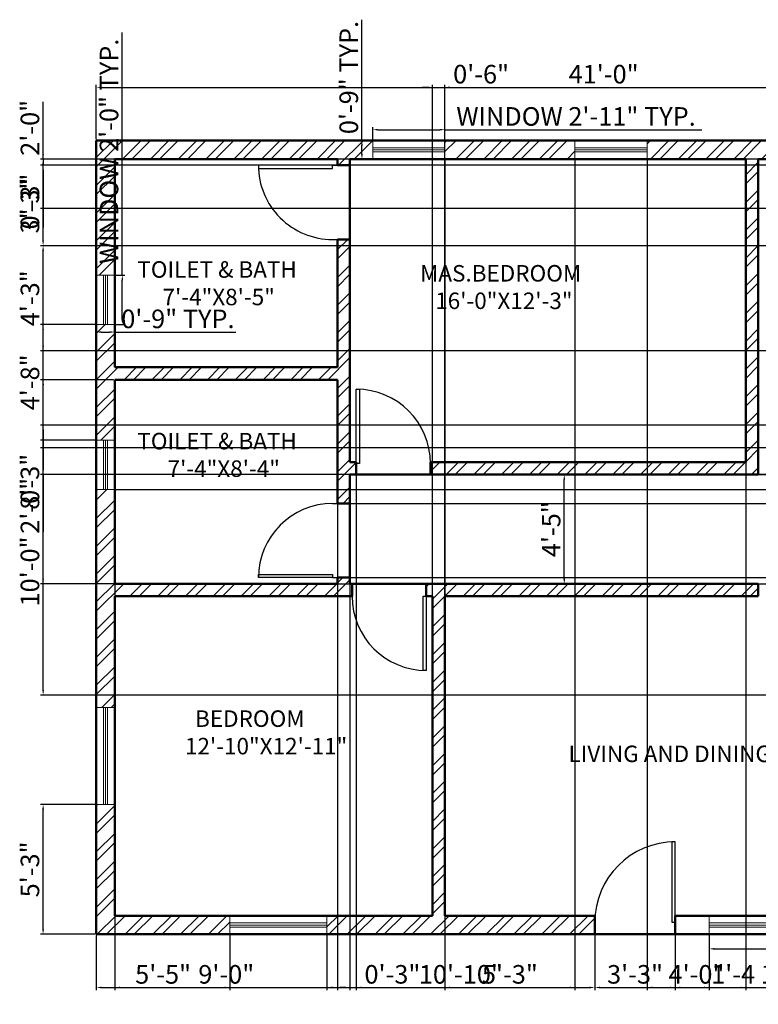
# Model space of a CAD drawing. Units: inches. Extents: x 935 to 4718, y 294 to 2318.
# Tile 1 of 2: x 935 to 1293, y 1841 to 2318. Entities that reach past the tile are written whole.
import ezdxf

# ---------------------------------------------------------------- set-up
doc = ezdxf.new("R2010")
doc.units = ezdxf.units.IN
for name, color, linetype, lineweight in [('A-ANNO-DIMS', 2, 'Continuous', 18), ('A-AREA-IDEN', 7, 'Continuous', 25), ('A-DOOR', 4, 'Continuous', 25), ('A-FLOR-CASE', 8, 'Continuous', 25), ('A-GLAZ', 244, 'Continuous', 18), ('A-WALL', 7, 'Continuous', 50), ('A-WALL-PATT', 8, 'Continuous', 13)]:
    doc.layers.add(name, color=color, linetype=linetype, lineweight=lineweight)
doc.styles.get("Standard").update_dxf_attribs({"font": 'arial.ttf'})
doc.dimstyles.new('ISO-25', dxfattribs={"dimtxt": 9, "dimasz": 2.5, "dimexe": 1.25, "dimexo": 0.625, "dimtad": 1, "dimlunit": 3, "dimtxsty": 'Standard', "dimcen": 2.5, "dimadec": 0, "dimazin": 0, "dimtfac": 1, "dimtmove": 0, "dimatfit": 3, "dimfxl": 1, "dimarcsym": 0})

# ---------------------------------------------------------------- blocks, each defined once
blk = doc.blocks.new('*U2')
for p, q in [((0, 0), (0, -6)), ((40, 0), (40, -6))]:
    blk.add_line(p, q)
blk.add_lwpolyline([(0, 0), (0, 40), (1.75, 40), (1.75, 0)], close=True)
blk.add_arc((0, 0), 40, 0, 90)
blk = doc.blocks.new('*U3')
for p, q in [((0, 0), (0, -6)), ((-40, 0), (-40, -6))]:
    blk.add_line(p, q)
blk.add_lwpolyline([(0, 0), (0, 40), (-1.75, 40), (-1.75, 0)], close=True)
blk.add_arc((0, 0), 40, 90, 180)
blk = doc.blocks.new('*U4')
for p, q in [((-40, 0), (-40, 6)), ((0, 0), (0, 6))]:
    blk.add_line(p, q)
blk.add_lwpolyline([(0, 0), (0, -40), (-1.75, -40), (-1.75, 0)], close=True)
blk.add_arc((0, 0), 40, 180, 270)
blk = doc.blocks.new('*U5')
for p, q in [((0, 0), (0, 6)), ((40, 0), (40, 6))]:
    blk.add_line(p, q)
blk.add_lwpolyline([(0, 0), (0, -40), (1.75, -40), (1.75, 0)], close=True)
blk.add_arc((0, 0), 40, 270, 0)
blk = doc.blocks.new('*D6')
at = {"layer": 'A-ANNO-DIMS', "color": 0, "lineweight": -2, "transparency": 16777216}
for p, q in [((1201.5, 2097.69), (1197.39, 2097.69)), ((1198.64, 2047.19), (1198.64, 2095.19)), ((1201.5, 2044.69), (1197.39, 2044.69))]:
    blk.add_line(p, q, dxfattribs=at)
at = {"layer": 'A-ANNO-DIMS', "color": 0, "transparency": 16777216}
for points in [[(1198.22, 2095.19), (1199.06, 2095.19), (1198.64, 2097.69)], [(1198.22, 2047.19), (1199.06, 2047.19), (1198.64, 2044.69)]]:
    blk.add_solid(points, dxfattribs=at)
at = {"layer": 'Defpoints', "color": 0, "transparency": 16777216}
for p in [(1198.64, 2097.69), (1202.12, 2097.69), (1202.12, 2044.69)]:
    blk.add_point(p, dxfattribs=at)
at = {"layer": 'A-ANNO-DIMS', "color": 0, "transparency": 16777216, "insert": (1193.44, 2071.19), "char_height": 9, "attachment_point": 5, "rotation": 90}
blk.add_mtext('4\'-5"', dxfattribs=at)
blk = doc.blocks.new('WIN-47IN')
for p, q in [((0, 5.5), (47, 5.5)), ((0, 4.5), (47, 4.5)), ((0, 3.5), (47, 3.5))]:
    blk.add_line(p, q)
blk.add_lwpolyline([(0, 9), (47, 9), (47, 0), (0, 0)], close=True)
blk = doc.blocks.new('WIN-35IN')
for p, q in [((0, 5.5), (35, 5.5)), ((0, 4.5), (35, 4.5)), ((0, 3.5), (35, 3.5))]:
    blk.add_line(p, q)
blk.add_lwpolyline([(0, 9), (35, 9), (35, 0), (0, 0)], close=True)
blk = doc.blocks.new('WIN-24IN')
for p, q in [((3.5, 24), (3.5, 0)), ((4.5, 24), (4.5, 0)), ((5.5, 24), (5.5, 0))]:
    blk.add_line(p, q)
blk.add_lwpolyline([(0, 24), (9, 24), (9, 0), (0, 0)], close=True)
blk = doc.blocks.new('*D10')
at = {"layer": 'A-ANNO-DIMS', "color": 0, "lineweight": -2, "transparency": 16777216}
for p, q in [((1268.86, 1874.07), (1268.86, 1866.39)), ((1315.86, 1874.07), (1315.86, 1866.39)), ((1271.36, 1867.64), (1313.36, 1867.64)), ((1315.86, 1867.64), (1440.49, 1867.64))]:
    blk.add_line(p, q, dxfattribs=at)
at = {"layer": 'A-ANNO-DIMS', "color": 0, "transparency": 16777216}
for points in [[(1271.36, 1868.06), (1271.36, 1867.23), (1268.86, 1867.64)], [(1313.36, 1868.06), (1313.36, 1867.23), (1315.86, 1867.64)]]:
    blk.add_solid(points, dxfattribs=at)
at = {"layer": 'Defpoints', "color": 0, "transparency": 16777216}
for p in [(1268.86, 1874.69), (1315.86, 1874.69), (1315.86, 1867.64)]:
    blk.add_point(p, dxfattribs=at)
at = {"layer": 'A-ANNO-DIMS', "color": 0, "transparency": 16777216, "insert": (1379.42, 1872.93), "char_height": 9, "attachment_point": 5}
blk.add_mtext('WINDOW 3\'-11" TYP.', dxfattribs=at)
blk = doc.blocks.new('*D12')
at = {"layer": 'A-ANNO-DIMS', "color": 0, "lineweight": -2, "transparency": 16777216}
for p, q in [((1105.77, 2260.32), (1105.77, 2266.19)), ((1108.27, 2264.94), (1138.27, 2264.94)), ((1140.77, 2260.32), (1140.77, 2266.19)), ((1140.77, 2264.94), (1265.4, 2264.94))]:
    blk.add_line(p, q, dxfattribs=at)
at = {"layer": 'A-ANNO-DIMS', "color": 0, "transparency": 16777216}
for points in [[(1108.27, 2265.36), (1108.27, 2264.53), (1105.77, 2264.94)], [(1138.27, 2265.36), (1138.27, 2264.53), (1140.77, 2264.94)]]:
    blk.add_solid(points, dxfattribs=at)
at = {"layer": 'Defpoints', "color": 0, "transparency": 16777216}
for p in [(1140.77, 2264.94), (1105.77, 2259.69), (1140.77, 2259.69)]:
    blk.add_point(p, dxfattribs=at)
at = {"layer": 'A-ANNO-DIMS', "color": 0, "transparency": 16777216, "insert": (1204.34, 2270.22), "char_height": 9, "attachment_point": 5}
blk.add_mtext('WINDOW 2\'-11" TYP.', dxfattribs=at)
blk = doc.blocks.new('*D13')
at = {"layer": 'A-ANNO-DIMS', "color": 0, "lineweight": -2, "transparency": 16777216}
for p, q in [((1100.52, 2259.69), (1100.52, 2318.3)), ((1105.15, 2259.69), (1099.27, 2259.69)), ((1100.52, 2253.19), (1100.52, 2257.19)), ((1105.15, 2250.69), (1099.27, 2250.69))]:
    blk.add_line(p, q, dxfattribs=at)
at = {"layer": 'A-ANNO-DIMS', "color": 0, "transparency": 16777216}
for points in [[(1100.1, 2257.19), (1100.94, 2257.19), (1100.52, 2259.69)], [(1100.1, 2253.19), (1100.94, 2253.19), (1100.52, 2250.69)]]:
    blk.add_solid(points, dxfattribs=at)
at = {"layer": 'Defpoints', "color": 0, "transparency": 16777216}
for p in [(1100.52, 2259.69), (1105.77, 2259.69), (1105.77, 2250.69)]:
    blk.add_point(p, dxfattribs=at)
at = {"layer": 'A-ANNO-DIMS', "color": 0, "transparency": 16777216, "insert": (1095.3, 2290.25), "char_height": 9, "attachment_point": 5, "rotation": 90}
blk.add_mtext('0\'-9" TYP.', dxfattribs=at)
blk = doc.blocks.new('*D14')
at = {"layer": 'A-ANNO-DIMS', "color": 0, "lineweight": -2, "transparency": 16777216}
for p, q in [((984.33, 2194.41), (984.33, 2312.04)), ((981.35, 2194.41), (985.58, 2194.41)), ((984.33, 2172.91), (984.33, 2191.91)), ((981.35, 2170.41), (985.58, 2170.41))]:
    blk.add_line(p, q, dxfattribs=at)
at = {"layer": 'A-ANNO-DIMS', "color": 0, "transparency": 16777216}
for points in [[(983.91, 2191.91), (984.74, 2191.91), (984.33, 2194.41)], [(983.91, 2172.91), (984.74, 2172.91), (984.33, 2170.41)]]:
    blk.add_solid(points, dxfattribs=at)
at = {"layer": 'Defpoints', "color": 0, "transparency": 16777216}
for p in [(980.73, 2194.41), (984.33, 2194.41), (980.73, 2170.41)]:
    blk.add_point(p, dxfattribs=at)
at = {"layer": 'A-ANNO-DIMS', "color": 0, "transparency": 16777216, "insert": (979.04, 2254.47), "char_height": 9, "attachment_point": 5, "rotation": 90}
blk.add_mtext('WINDOW 2\'-0" TYP.', dxfattribs=at)
blk = doc.blocks.new('*D15')
at = {"layer": 'A-ANNO-DIMS', "color": 0, "lineweight": -2, "transparency": 16777216}
for p, q in [((971.73, 2169.78), (971.73, 2165.56)), ((980.73, 2169.78), (980.73, 2165.56)), ((974.23, 2166.81), (978.23, 2166.81)), ((980.73, 2166.81), (1039.33, 2166.81))]:
    blk.add_line(p, q, dxfattribs=at)
at = {"layer": 'A-ANNO-DIMS', "color": 0, "transparency": 16777216}
for points in [[(974.23, 2167.22), (974.23, 2166.39), (971.73, 2166.81)], [(978.23, 2167.22), (978.23, 2166.39), (980.73, 2166.81)]]:
    blk.add_solid(points, dxfattribs=at)
at = {"layer": 'Defpoints', "color": 0, "transparency": 16777216}
for p in [(971.73, 2170.41), (980.73, 2170.41), (980.73, 2166.81)]:
    blk.add_point(p, dxfattribs=at)
at = {"layer": 'A-ANNO-DIMS', "color": 0, "transparency": 16777216, "insert": (1011.28, 2172.03), "char_height": 9, "attachment_point": 5}
blk.add_mtext('0\'-9" TYP.', dxfattribs=at)
blk = doc.blocks.new('*D16')
at = {"layer": 'A-ANNO-DIMS', "color": 0, "lineweight": -2, "transparency": 16777216}
for p, q in [((971.73, 2260.32), (971.73, 2286.74)), ((974.23, 2285.49), (1461.23, 2285.49)), ((1463.73, 2260.32), (1463.73, 2286.74))]:
    blk.add_line(p, q, dxfattribs=at)
at = {"layer": 'A-ANNO-DIMS', "color": 0, "transparency": 16777216}
for points in [[(974.23, 2285.91), (974.23, 2285.08), (971.73, 2285.49)], [(1461.23, 2285.91), (1461.23, 2285.08), (1463.73, 2285.49)]]:
    blk.add_solid(points, dxfattribs=at)
at = {"layer": 'Defpoints', "color": 0, "transparency": 16777216}
for p in [(1463.73, 2285.49), (971.73, 2259.69), (1463.73, 2259.69)]:
    blk.add_point(p, dxfattribs=at)
at = {"layer": 'A-ANNO-DIMS', "color": 0, "transparency": 16777216, "insert": (1217.73, 2290.71), "char_height": 9, "attachment_point": 5}
blk.add_mtext('41\'-0"', dxfattribs=at)
blk = doc.blocks.new('*D18')
at = {"layer": 'A-ANNO-DIMS', "color": 0, "lineweight": -2, "transparency": 16777216}
for p, q in [((1140.77, 2250.07), (1140.77, 1847.64)), ((1203.77, 2250.07), (1203.77, 1847.64)), ((1143.27, 1848.89), (1201.27, 1848.89))]:
    blk.add_line(p, q, dxfattribs=at)
at = {"layer": 'A-ANNO-DIMS', "color": 0, "transparency": 16777216}
for points in [[(1143.27, 1849.31), (1143.27, 1848.48), (1140.77, 1848.89)], [(1201.27, 1849.31), (1201.27, 1848.48), (1203.77, 1848.89)]]:
    blk.add_solid(points, dxfattribs=at)
at = {"layer": 'Defpoints', "color": 0, "transparency": 16777216}
for p in [(1140.77, 2250.69), (1203.77, 2250.69), (1203.77, 1848.89)]:
    blk.add_point(p, dxfattribs=at)
at = {"layer": 'A-ANNO-DIMS', "color": 0, "transparency": 16777216, "insert": (1172.27, 1854.12), "char_height": 9, "attachment_point": 5}
blk.add_mtext('5\'-3"', dxfattribs=at)
blk = doc.blocks.new('*D19')
at = {"layer": 'A-ANNO-DIMS', "color": 0, "lineweight": -2, "transparency": 16777216}
for p, q in [((1238.77, 2250.07), (1238.77, 1847.64)), ((1286.73, 2250.07), (1286.73, 1847.64)), ((1241.27, 1848.89), (1284.23, 1848.89))]:
    blk.add_line(p, q, dxfattribs=at)
at = {"layer": 'A-ANNO-DIMS', "color": 0, "transparency": 16777216}
for points in [[(1241.27, 1849.31), (1241.27, 1848.48), (1238.77, 1848.89)], [(1284.23, 1849.31), (1284.23, 1848.48), (1286.73, 1848.89)]]:
    blk.add_solid(points, dxfattribs=at)
at = {"layer": 'Defpoints', "color": 0, "transparency": 16777216}
for p in [(1238.77, 2250.69), (1286.73, 2250.69), (1286.73, 1848.89)]:
    blk.add_point(p, dxfattribs=at)
at = {"layer": 'A-ANNO-DIMS', "color": 0, "transparency": 16777216, "insert": (1262.75, 1854.11), "char_height": 9, "attachment_point": 5}
blk.add_mtext('4\'-0"', dxfattribs=at)
blk = doc.blocks.new('*D21')
at = {"layer": 'A-ANNO-DIMS', "color": 0, "lineweight": -2, "transparency": 16777216}
for p, q in [((971.73, 1874.07), (971.73, 1847.64)), ((1036.52, 1874.07), (1036.52, 1847.64)), ((974.23, 1848.89), (1034.02, 1848.89))]:
    blk.add_line(p, q, dxfattribs=at)
at = {"layer": 'A-ANNO-DIMS', "color": 0, "transparency": 16777216}
for points in [[(974.23, 1849.31), (974.23, 1848.48), (971.73, 1848.89)], [(1034.02, 1849.31), (1034.02, 1848.48), (1036.52, 1848.89)]]:
    blk.add_solid(points, dxfattribs=at)
at = {"layer": 'Defpoints', "color": 0, "transparency": 16777216}
for p in [(971.73, 1874.69), (1036.52, 1874.69), (1036.52, 1848.89)]:
    blk.add_point(p, dxfattribs=at)
at = {"layer": 'A-ANNO-DIMS', "color": 0, "transparency": 16777216, "insert": (1004.12, 1854.09), "char_height": 9, "attachment_point": 5}
blk.add_mtext('5\'-5"', dxfattribs=at)
blk = doc.blocks.new('*D22')
at = {"layer": 'A-ANNO-DIMS', "color": 0, "lineweight": -2, "transparency": 16777216}
for p, q in [((1083.52, 1874.07), (1083.52, 1847.64)), ((1213.46, 1874.07), (1213.46, 1847.64)), ((1086.02, 1848.89), (1210.96, 1848.89))]:
    blk.add_line(p, q, dxfattribs=at)
at = {"layer": 'A-ANNO-DIMS', "color": 0, "transparency": 16777216}
for points in [[(1086.02, 1849.31), (1086.02, 1848.48), (1083.52, 1848.89)], [(1210.96, 1849.31), (1210.96, 1848.48), (1213.46, 1848.89)]]:
    blk.add_solid(points, dxfattribs=at)
at = {"layer": 'Defpoints', "color": 0, "transparency": 16777216}
for p in [(1083.52, 1874.69), (1213.46, 1874.69), (1213.46, 1848.89)]:
    blk.add_point(p, dxfattribs=at)
at = {"layer": 'A-ANNO-DIMS', "color": 0, "transparency": 16777216, "insert": (1148.49, 1854.11), "char_height": 9, "attachment_point": 5}
blk.add_mtext('10\'-10"', dxfattribs=at)
blk = doc.blocks.new('*D23')
at = {"layer": 'A-ANNO-DIMS', "color": 0, "lineweight": -2, "transparency": 16777216}
for p, q in [((1213.46, 1874.07), (1213.46, 1847.64)), ((1252.46, 1874.07), (1252.46, 1847.64)), ((1215.96, 1848.89), (1249.96, 1848.89))]:
    blk.add_line(p, q, dxfattribs=at)
at = {"layer": 'A-ANNO-DIMS', "color": 0, "transparency": 16777216}
for points in [[(1215.96, 1849.31), (1215.96, 1848.48), (1213.46, 1848.89)], [(1249.96, 1849.31), (1249.96, 1848.48), (1252.46, 1848.89)]]:
    blk.add_solid(points, dxfattribs=at)
at = {"layer": 'Defpoints', "color": 0, "transparency": 16777216}
for p in [(1213.46, 1874.69), (1252.46, 1874.69), (1252.46, 1848.89)]:
    blk.add_point(p, dxfattribs=at)
at = {"layer": 'A-ANNO-DIMS', "color": 0, "transparency": 16777216, "insert": (1232.96, 1854.12), "char_height": 9, "attachment_point": 5}
blk.add_mtext('3\'-3"', dxfattribs=at)
blk = doc.blocks.new('*D24')
at = {"layer": 'A-ANNO-DIMS', "color": 0, "lineweight": -2, "transparency": 16777216}
for p, q in [((1252.46, 1874.07), (1252.46, 1847.64)), ((1268.86, 1874.07), (1268.86, 1847.64)), ((1254.96, 1848.89), (1266.36, 1848.89)), ((1268.86, 1848.89), (1316.66, 1848.89))]:
    blk.add_line(p, q, dxfattribs=at)
at = {"layer": 'A-ANNO-DIMS', "color": 0, "transparency": 16777216}
for points in [[(1254.96, 1849.31), (1254.96, 1848.48), (1252.46, 1848.89)], [(1266.36, 1849.31), (1266.36, 1848.48), (1268.86, 1848.89)]]:
    blk.add_solid(points, dxfattribs=at)
at = {"layer": 'Defpoints', "color": 0, "transparency": 16777216}
for p in [(1252.46, 1874.69), (1268.86, 1874.69), (1268.86, 1848.89)]:
    blk.add_point(p, dxfattribs=at)
at = {"layer": 'A-ANNO-DIMS', "color": 0, "transparency": 16777216, "insert": (1294.01, 1854.17), "char_height": 9, "attachment_point": 5}
blk.add_mtext('1\'-4 1/2"', dxfattribs=at)
blk = doc.blocks.new('*D26')
at = {"layer": 'A-ANNO-DIMS', "color": 0, "lineweight": -2, "transparency": 16777216}
for p, q in [((971.1, 1937.69), (944.68, 1937.69)), ((945.93, 1877.19), (945.93, 1935.19)), ((971.1, 1874.69), (944.68, 1874.69))]:
    blk.add_line(p, q, dxfattribs=at)
at = {"layer": 'A-ANNO-DIMS', "color": 0, "transparency": 16777216}
for points in [[(945.51, 1935.19), (946.34, 1935.19), (945.93, 1937.69)], [(945.51, 1877.19), (946.34, 1877.19), (945.93, 1874.69)]]:
    blk.add_solid(points, dxfattribs=at)
at = {"layer": 'Defpoints', "color": 0, "transparency": 16777216}
for p in [(945.93, 1937.69), (971.73, 1937.69), (971.73, 1874.69)]:
    blk.add_point(p, dxfattribs=at)
at = {"layer": 'A-ANNO-DIMS', "color": 0, "transparency": 16777216, "insert": (940.7, 1906.19), "char_height": 9, "attachment_point": 5, "rotation": 90}
blk.add_mtext('5\'-3"', dxfattribs=at)
blk = doc.blocks.new('*D27')
at = {"layer": 'A-ANNO-DIMS', "color": 0, "lineweight": -2, "transparency": 16777216}
for p, q in [((1489.53, 2090.41), (1489.53, 2139.04)), ((981.35, 2090.41), (1490.78, 2090.41)), ((1489.53, 2047.19), (1489.53, 2087.91)), ((981.35, 2044.69), (1490.78, 2044.69))]:
    blk.add_line(p, q, dxfattribs=at)
at = {"layer": 'A-ANNO-DIMS', "color": 0, "transparency": 16777216}
for points in [[(1489.11, 2087.91), (1489.94, 2087.91), (1489.53, 2090.41)], [(1489.11, 2047.19), (1489.94, 2047.19), (1489.53, 2044.69)]]:
    blk.add_solid(points, dxfattribs=at)
at = {"layer": 'Defpoints', "color": 0, "transparency": 16777216}
for p in [(980.73, 2090.41), (1489.53, 2090.41), (980.73, 2044.69)]:
    blk.add_point(p, dxfattribs=at)
at = {"layer": 'A-ANNO-DIMS', "color": 0, "transparency": 16777216, "insert": (1484.24, 2115.97), "char_height": 9, "attachment_point": 5, "rotation": 90}
blk.add_mtext('3\'-9 1/2"', dxfattribs=at)
blk = doc.blocks.new('*D28')
at = {"layer": 'A-ANNO-DIMS', "color": 0, "lineweight": -2, "transparency": 16777216}
for p, q in [((971.1, 2170.41), (944.68, 2170.41)), ((945.93, 2116.91), (945.93, 2167.91)), ((971.1, 2114.41), (944.68, 2114.41))]:
    blk.add_line(p, q, dxfattribs=at)
at = {"layer": 'A-ANNO-DIMS', "color": 0, "transparency": 16777216}
for points in [[(945.51, 2167.91), (946.34, 2167.91), (945.93, 2170.41)], [(945.51, 2116.91), (946.34, 2116.91), (945.93, 2114.41)]]:
    blk.add_solid(points, dxfattribs=at)
at = {"layer": 'Defpoints', "color": 0, "transparency": 16777216}
for p in [(945.93, 2170.41), (971.73, 2170.41), (971.73, 2114.41)]:
    blk.add_point(p, dxfattribs=at)
at = {"layer": 'A-ANNO-DIMS', "color": 0, "transparency": 16777216, "insert": (940.7, 2142.41), "char_height": 9, "attachment_point": 5, "rotation": 90}
blk.add_mtext('4\'-8"', dxfattribs=at)
blk = doc.blocks.new('*D29')
at = {"layer": 'A-ANNO-DIMS', "color": 0, "lineweight": -2, "transparency": 16777216}
for p, q in [((945.93, 2253.19), (945.93, 2255.69)), ((1454.1, 2250.69), (944.68, 2250.69)), ((945.93, 2250.69), (945.93, 2247.69)), ((1418.25, 2247.69), (944.68, 2247.69)), ((945.93, 2245.19), (945.93, 2217.52))]:
    blk.add_line(p, q, dxfattribs=at)
at = {"layer": 'A-ANNO-DIMS', "color": 0, "transparency": 16777216}
for points in [[(945.51, 2253.19), (946.34, 2253.19), (945.93, 2250.69)], [(945.51, 2245.19), (946.34, 2245.19), (945.93, 2247.69)]]:
    blk.add_solid(points, dxfattribs=at)
at = {"layer": 'Defpoints', "color": 0, "transparency": 16777216}
for p in [(1454.73, 2250.69), (945.93, 2247.69), (1418.88, 2247.69)]:
    blk.add_point(p, dxfattribs=at)
at = {"layer": 'A-ANNO-DIMS', "color": 0, "transparency": 16777216, "insert": (940.7, 2230.11), "char_height": 9, "attachment_point": 5, "rotation": 90}
blk.add_mtext('0\'-3"', dxfattribs=at)
blk = doc.blocks.new('*D30')
at = {"layer": 'A-ANNO-DIMS', "color": 0, "lineweight": -2, "transparency": 16777216}
for p, q in [((1454.1, 2110.69), (944.68, 2110.69)), ((945.93, 1993.19), (945.93, 2108.19)), ((1454.1, 1990.69), (944.68, 1990.69))]:
    blk.add_line(p, q, dxfattribs=at)
at = {"layer": 'A-ANNO-DIMS', "color": 0, "transparency": 16777216}
for points in [[(945.51, 2108.19), (946.34, 2108.19), (945.93, 2110.69)], [(945.51, 1993.19), (946.34, 1993.19), (945.93, 1990.69)]]:
    blk.add_solid(points, dxfattribs=at)
at = {"layer": 'Defpoints', "color": 0, "transparency": 16777216}
for p in [(945.93, 2110.69), (1454.73, 2110.69), (1454.73, 1990.69)]:
    blk.add_point(p, dxfattribs=at)
at = {"layer": 'A-ANNO-DIMS', "color": 0, "transparency": 16777216, "insert": (940.7, 2050.69), "char_height": 9, "attachment_point": 5, "rotation": 90}
blk.add_mtext('10\'-0"', dxfattribs=at)
blk = doc.blocks.new('*D31')
at = {"layer": 'A-ANNO-DIMS', "color": 0, "lineweight": -2, "transparency": 16777216}
for p, q in [((1454.1, 2208.69), (944.68, 2208.69)), ((945.93, 2160.19), (945.93, 2206.19)), ((1454.1, 2157.69), (944.68, 2157.69))]:
    blk.add_line(p, q, dxfattribs=at)
at = {"layer": 'A-ANNO-DIMS', "color": 0, "transparency": 16777216}
for points in [[(945.51, 2206.19), (946.34, 2206.19), (945.93, 2208.69)], [(945.51, 2160.19), (946.34, 2160.19), (945.93, 2157.69)]]:
    blk.add_solid(points, dxfattribs=at)
at = {"layer": 'Defpoints', "color": 0, "transparency": 16777216}
for p in [(945.93, 2208.69), (1454.73, 2208.69), (1454.73, 2157.69)]:
    blk.add_point(p, dxfattribs=at)
at = {"layer": 'A-ANNO-DIMS', "color": 0, "transparency": 16777216, "insert": (940.7, 2183.19), "char_height": 9, "attachment_point": 5, "rotation": 90}
blk.add_mtext('4\'-3"', dxfattribs=at)
blk = doc.blocks.new('*D32')
at = {"layer": 'A-ANNO-DIMS', "color": 0, "lineweight": -2, "transparency": 16777216}
for p, q in [((1454.1, 2247.69), (944.68, 2247.69)), ((945.93, 2211.19), (945.93, 2245.19)), ((1454.1, 2208.69), (944.68, 2208.69))]:
    blk.add_line(p, q, dxfattribs=at)
at = {"layer": 'A-ANNO-DIMS', "color": 0, "transparency": 16777216}
for points in [[(945.51, 2245.19), (946.34, 2245.19), (945.93, 2247.69)], [(945.51, 2211.19), (946.34, 2211.19), (945.93, 2208.69)]]:
    blk.add_solid(points, dxfattribs=at)
at = {"layer": 'Defpoints', "color": 0, "transparency": 16777216}
for p in [(945.93, 2247.69), (1454.73, 2247.69), (1454.73, 2208.69)]:
    blk.add_point(p, dxfattribs=at)
at = {"layer": 'A-ANNO-DIMS', "color": 0, "transparency": 16777216, "insert": (940.7, 2228.19), "char_height": 9, "attachment_point": 5, "rotation": 90}
blk.add_mtext('3\'-3"', dxfattribs=at)
blk = doc.blocks.new('*D33')
at = {"layer": 'A-ANNO-DIMS', "color": 0, "lineweight": -2, "transparency": 16777216}
for p, q in [((980.73, 2143.07), (980.73, 1847.64)), ((1088.73, 2143.07), (1088.73, 1847.64)), ((983.23, 1848.89), (1086.23, 1848.89))]:
    blk.add_line(p, q, dxfattribs=at)
at = {"layer": 'A-ANNO-DIMS', "color": 0, "transparency": 16777216}
for points in [[(983.23, 1849.31), (983.23, 1848.48), (980.73, 1848.89)], [(1086.23, 1849.31), (1086.23, 1848.48), (1088.73, 1848.89)]]:
    blk.add_solid(points, dxfattribs=at)
at = {"layer": 'Defpoints', "color": 0, "transparency": 16777216}
for p in [(980.73, 2143.69), (1088.73, 2143.69), (1088.73, 1848.89)]:
    blk.add_point(p, dxfattribs=at)
at = {"layer": 'A-ANNO-DIMS', "color": 0, "transparency": 16777216, "insert": (1034.73, 1854.11), "char_height": 9, "attachment_point": 5}
blk.add_mtext('9\'-0"', dxfattribs=at)
blk = doc.blocks.new('*D34')
at = {"layer": 'A-ANNO-DIMS', "color": 0, "lineweight": -2, "transparency": 16777216}
for p, q in [((980.1, 2143.69), (944.68, 2143.69)), ((945.93, 2047.19), (945.93, 2141.19)), ((980.1, 2044.69), (944.68, 2044.69))]:
    blk.add_line(p, q, dxfattribs=at)
at = {"layer": 'A-ANNO-DIMS', "color": 0, "transparency": 16777216}
for points in [[(945.51, 2141.19), (946.34, 2141.19), (945.93, 2143.69)], [(945.51, 2047.19), (946.34, 2047.19), (945.93, 2044.69)]]:
    blk.add_solid(points, dxfattribs=at)
at = {"layer": 'Defpoints', "color": 0, "transparency": 16777216}
for p in [(945.93, 2143.69), (980.73, 2143.69), (980.73, 2044.69)]:
    blk.add_point(p, dxfattribs=at)
at = {"layer": 'A-ANNO-DIMS', "color": 0, "transparency": 16777216, "insert": (940.7, 2094.19), "char_height": 9, "attachment_point": 5, "rotation": 90}
blk.add_mtext('8\'-3"', dxfattribs=at)
blk = doc.blocks.new('*D35')
at = {"layer": 'A-ANNO-DIMS', "color": 0, "lineweight": -2, "transparency": 16777216}
for p, q in [((1132.23, 2285.49), (1129.73, 2285.49)), ((1134.73, 1884.32), (1134.73, 2286.74)), ((1134.73, 2285.49), (1140.73, 2285.49)), ((1140.73, 1884.32), (1140.73, 2286.74)), ((1143.23, 2285.49), (1170.9, 2285.49))]:
    blk.add_line(p, q, dxfattribs=at)
at = {"layer": 'A-ANNO-DIMS', "color": 0, "transparency": 16777216}
for points in [[(1132.23, 2285.91), (1132.23, 2285.08), (1134.73, 2285.49)], [(1143.23, 2285.91), (1143.23, 2285.08), (1140.73, 2285.49)]]:
    blk.add_solid(points, dxfattribs=at)
at = {"layer": 'Defpoints', "color": 0, "transparency": 16777216}
for p in [(1140.73, 2285.49), (1134.73, 1883.69), (1140.73, 1883.69)]:
    blk.add_point(p, dxfattribs=at)
at = {"layer": 'A-ANNO-DIMS', "color": 0, "transparency": 16777216, "insert": (1158.31, 2290.71), "char_height": 9, "attachment_point": 5}
blk.add_mtext('0\'-6"', dxfattribs=at)
blk = doc.blocks.new('*D37')
at = {"layer": 'A-ANNO-DIMS', "color": 0, "lineweight": -2, "transparency": 16777216}
for p, q in [((945.93, 2250.69), (945.93, 2278.52)), ((1391.1, 2250.69), (944.68, 2250.69)), ((945.93, 2229.19), (945.93, 2248.19)), ((1391.1, 2226.69), (944.68, 2226.69))]:
    blk.add_line(p, q, dxfattribs=at)
at = {"layer": 'A-ANNO-DIMS', "color": 0, "transparency": 16777216}
for points in [[(945.51, 2248.19), (946.34, 2248.19), (945.93, 2250.69)], [(945.51, 2229.19), (946.34, 2229.19), (945.93, 2226.69)]]:
    blk.add_solid(points, dxfattribs=at)
at = {"layer": 'Defpoints', "color": 0, "transparency": 16777216}
for p in [(945.93, 2250.69), (1391.73, 2250.69), (1391.73, 2226.69)]:
    blk.add_point(p, dxfattribs=at)
at = {"layer": 'A-ANNO-DIMS', "color": 0, "transparency": 16777216, "insert": (940.7, 2265.86), "char_height": 9, "attachment_point": 5, "rotation": 90}
blk.add_mtext('2\'-0"', dxfattribs=at)
blk = doc.blocks.new('*D41')
at = {"layer": 'A-ANNO-DIMS', "color": 0, "lineweight": -2, "transparency": 16777216}
for p, q in [((1358.25, 2121.69), (944.68, 2121.69)), ((945.93, 2119.19), (945.93, 2100.19)), ((1358.25, 2097.69), (944.68, 2097.69)), ((945.93, 2097.69), (945.93, 2069.87))]:
    blk.add_line(p, q, dxfattribs=at)
at = {"layer": 'A-ANNO-DIMS', "color": 0, "transparency": 16777216}
for points in [[(945.51, 2119.19), (946.34, 2119.19), (945.93, 2121.69)], [(945.51, 2100.19), (946.34, 2100.19), (945.93, 2097.69)]]:
    blk.add_solid(points, dxfattribs=at)
at = {"layer": 'Defpoints', "color": 0, "transparency": 16777216}
for p in [(1358.88, 2121.69), (945.93, 2097.69), (1358.88, 2097.69)]:
    blk.add_point(p, dxfattribs=at)
at = {"layer": 'A-ANNO-DIMS', "color": 0, "transparency": 16777216, "insert": (940.7, 2082.53), "char_height": 9, "attachment_point": 5, "rotation": 90}
blk.add_mtext('2\'-0"', dxfattribs=at)
blk = doc.blocks.new('*D42')
at = {"layer": 'A-ANNO-DIMS', "color": 0, "lineweight": -2, "transparency": 16777216}
for p, q in [((1095.35, 2083.69), (1490.78, 2083.69)), ((1489.53, 2050.19), (1489.53, 2081.19)), ((1095.35, 2047.69), (1490.78, 2047.69))]:
    blk.add_line(p, q, dxfattribs=at)
at = {"layer": 'A-ANNO-DIMS', "color": 0, "transparency": 16777216}
for points in [[(1489.11, 2081.19), (1489.94, 2081.19), (1489.53, 2083.69)], [(1489.11, 2050.19), (1489.94, 2050.19), (1489.53, 2047.69)]]:
    blk.add_solid(points, dxfattribs=at)
at = {"layer": 'Defpoints', "color": 0, "transparency": 16777216}
for p in [(1094.73, 2083.69), (1489.53, 2083.69), (1094.73, 2047.69)]:
    blk.add_point(p, dxfattribs=at)
at = {"layer": 'A-ANNO-DIMS', "color": 0, "transparency": 16777216, "insert": (1484.3, 2065.69), "char_height": 9, "attachment_point": 5, "rotation": 90}
blk.add_mtext('3\'-0"', dxfattribs=at)
blk = doc.blocks.new('*D43')
at = {"layer": 'A-ANNO-DIMS', "color": 0, "lineweight": -2, "transparency": 16777216}
for p, q in [((1094.73, 2097.07), (1094.73, 1847.64)), ((1097.73, 2097.07), (1097.73, 1847.64)), ((1092.23, 1848.89), (1089.73, 1848.89)), ((1094.73, 1848.89), (1097.73, 1848.89)), ((1100.23, 1848.89), (1127.9, 1848.89))]:
    blk.add_line(p, q, dxfattribs=at)
at = {"layer": 'A-ANNO-DIMS', "color": 0, "transparency": 16777216}
for points in [[(1092.23, 1849.31), (1092.23, 1848.48), (1094.73, 1848.89)], [(1100.23, 1849.31), (1100.23, 1848.48), (1097.73, 1848.89)]]:
    blk.add_solid(points, dxfattribs=at)
at = {"layer": 'Defpoints', "color": 0, "transparency": 16777216}
for p in [(1094.73, 2097.69), (1097.73, 2097.69), (1097.73, 1848.89)]:
    blk.add_point(p, dxfattribs=at)
at = {"layer": 'A-ANNO-DIMS', "color": 0, "transparency": 16777216, "insert": (1115.31, 1854.12), "char_height": 9, "attachment_point": 5}
blk.add_mtext('0\'-3"', dxfattribs=at)

msp = doc.modelspace()

# ---------------------------------------------------------------- hatches: boundary and pattern name
at = {"layer": 'A-WALL-PATT'}
h = msp.add_hatch(dxfattribs=at)
h.set_pattern_fill('ANSI32', color=256)
h.paths.add_polyline_path([(1292.725, 2044.693), (1131.725, 2044.693), (1131.725, 2038.693), (1134.725, 2038.693), (1134.725, 1883.693), (1083.516, 1883.693), (1083.516, 1874.693), (1213.462, 1874.693), (1213.462, 1883.693), (1140.725, 1883.693), (1140.725, 2038.693), (1292.725, 2038.693)])
h.paths.add_polyline_path([(1463.725, 1943.693), (1454.725, 1943.693), (1454.725, 1883.693), (1418.857, 1883.693), (1418.857, 1874.693), (1463.725, 1874.693)])
h.paths.add_polyline_path([(1463.725, 2110.693), (1454.725, 2110.693), (1454.725, 1990.693), (1463.725, 1990.693)])
h.paths.add_polyline_path([(1371.857, 1883.693), (1315.857, 1883.693), (1315.857, 1874.693), (1371.857, 1874.693)])
h.paths.add_polyline_path([(1036.516, 1883.693), (980.725, 1883.693), (980.725, 1937.693), (971.725, 1937.693), (971.725, 1874.693), (1036.516, 1874.693)])
h.paths.add_polyline_path([(980.725, 2038.693), (1094.725, 2038.693), (1095.725, 2038.693), (1095.725, 2044.093), (1095.725, 2044.693), (1094.725, 2044.693), (1094.725, 2047.693), (1088.725, 2047.693), (1088.725, 2044.693), (980.725, 2044.693), (980.725, 2090.405), (971.725, 2090.405), (971.725, 1984.693), (980.725, 1984.693)])
h.paths.add_polyline_path([(1292.725, 2250.693), (1348.753, 2250.693), (1348.753, 2259.693), (1238.771, 2259.693), (1238.771, 2250.693), (1286.725, 2250.693), (1286.725, 2103.693), (1133.725, 2103.693), (1133.725, 2097.693), (1292.725, 2097.693)])
h.paths.add_polyline_path([(1463.725, 2208.693), (1457.875, 2208.693), (1454.725, 2208.693), (1454.725, 2157.693), (1463.725, 2157.693)])
h.paths.add_polyline_path([(1463.725, 2259.693), (1395.753, 2259.693), (1395.753, 2250.693), (1454.725, 2250.693), (1454.725, 2247.693), (1457.875, 2247.693), (1463.725, 2247.693)])
h.paths.add_polyline_path([(1203.771, 2259.693), (1140.771, 2259.693), (1140.771, 2250.693), (1203.771, 2250.693)], flags=17)
h.paths.add_polyline_path([(1105.771, 2259.693), (971.725, 2259.693), (971.725, 2194.405), (980.725, 2194.405), (980.725, 2250.693), (1088.725, 2250.693), (1088.725, 2247.693), (1091.725, 2247.693), (1094.725, 2247.693), (1094.725, 2250.693), (1105.771, 2250.693)])
h.paths.add_polyline_path([(1094.725, 2211.693), (1088.725, 2211.693), (1088.725, 2149.693), (980.725, 2149.693), (980.725, 2170.405), (971.725, 2170.405), (971.725, 2114.405), (980.725, 2114.405), (980.725, 2143.693), (1088.725, 2143.693), (1088.725, 2083.693), (1091.725, 2083.693), (1094.725, 2083.693), (1094.725, 2097.693), (1097.725, 2097.693), (1097.725, 2103.693), (1094.725, 2103.693)])

# ---------------------------------------------------------------- linework, layer by layer
at = {"layer": 'A-FLOR-CASE'}
msp.add_line((1292.725, 2097.693), (1360.876, 2097.693), dxfattribs=at)
at = {"layer": 'A-WALL'}
for p, q in [((971.725, 2259.693), (971.725, 1874.693)), ((971.725, 2259.693), (1463.725, 2259.693)), ((980.725, 2250.693), (980.725, 2149.693)), ((980.725, 2250.693), (1088.725, 2250.693)), ((1088.725, 2250.693), (1088.725, 2247.693)), ((1094.725, 2250.693), (1094.725, 2103.693)), ((1094.725, 2250.693), (1286.725, 2250.693)), ((1286.725, 2250.693), (1286.725, 2103.693)), ((1292.725, 2250.693), (1292.725, 2097.693)), ((1292.725, 2250.693), (1454.725, 2250.693)), ((1094.725, 2247.693), (1088.725, 2247.693)), ((1094.725, 2211.693), (1088.725, 2211.693)), ((1088.725, 2211.693), (1088.725, 2149.693)), ((980.725, 2149.693), (1088.725, 2149.693)), ((980.725, 2143.693), (1088.725, 2143.693)), ((980.725, 2143.693), (980.725, 2044.693)), ((1088.725, 2143.693), (1088.725, 2083.693)), ((1094.725, 2103.693), (1097.725, 2103.693)), ((1097.725, 2103.693), (1097.725, 2097.693)), ((1133.725, 2103.693), (1133.725, 2097.693)), ((1133.725, 2103.693), (1286.725, 2103.693)), ((1094.725, 2097.693), (1292.725, 2097.693)), ((1094.725, 2097.693), (1094.725, 2044.693)), ((1094.725, 2083.693), (1088.725, 2083.693)), ((980.725, 2044.693), (1088.725, 2044.693)), ((1094.725, 2047.693), (1088.725, 2047.693)), ((1088.725, 2047.693), (1088.725, 2044.693)), ((1094.725, 2044.693), (1292.725, 2044.693)), ((1095.725, 2038.693), (1095.725, 2044.693)), ((1131.725, 2038.693), (1131.725, 2044.693)), ((1292.725, 2044.693), (1292.725, 2038.693)), ((980.725, 2038.693), (1094.725, 2038.693)), ((980.725, 2038.693), (980.725, 1883.693)), ((1094.725, 2038.693), (1095.725, 2038.693)), ((1131.725, 2038.693), (1134.725, 2038.693)), ((1134.725, 2038.693), (1134.725, 1883.693)), ((1140.725, 2038.693), (1140.725, 1883.693)), ((1140.725, 2038.693), (1292.725, 2038.693)), ((980.725, 1883.693), (1134.725, 1883.693)), ((1140.725, 1883.693), (1213.462, 1883.693)), ((1213.462, 1883.693), (1213.462, 1874.693)), ((1252.462, 1883.693), (1252.462, 1874.693)), ((1252.462, 1883.693), (1454.725, 1883.693)), ((971.725, 1874.693), (1463.725, 1874.693))]:
    msp.add_line(p, q, dxfattribs=at)

# ---------------------------------------------------------------- block references
at = {"layer": 'A-DOOR', "xscale": 0.9, "yscale": 0.9, "zscale": 0.9, "rotation": 270}
for name, p in [('*U5', (1086.325, 2247.693)), ('*U4', (1086.325, 2047.693))]:
    msp.add_blockref(name, p, dxfattribs=at)
at = {"layer": 'A-DOOR'}
for name, p, xscale, yscale, zscale in [('*U2', (1097.725, 2103.093), 0.9, 0.9, 0.9), ('*U4', (1131.725, 2038.693), 0.9, 0.9, 0.9), ('*U3', (1252.462, 1880.543), 0.975, 0.975, 0.975)]:
    msp.add_blockref(name, p, dxfattribs=dict(at, xscale=xscale, yscale=yscale, zscale=zscale))
at = {"layer": 'A-GLAZ'}
for name, p in [('WIN-35IN', (1105.771, 2250.693)), ('WIN-35IN', (1203.771, 2250.693)), ('WIN-24IN', (971.725, 2170.405)), ('WIN-24IN', (971.725, 2090.405)), ('WIN-47IN', (1036.516, 1874.693)), ('WIN-47IN', (1268.857, 1874.693))]:
    msp.add_blockref(name, p, dxfattribs=at)
at = {"layer": 'A-GLAZ', "rotation": 90.00000000000055}
msp.add_blockref('WIN-47IN', (980.725, 1937.693), dxfattribs=at)

# ---------------------------------------------------------------- texts
at = {"layer": 'A-AREA-IDEN', "char_height": 8, "attachment_point": 1}
for s, width, insert in [('TOILET & BATH\\P     7\'-4"X8\'-5"', 88.2028, (991.613, 2201.143)), ('MAS.BEDROOM\\P   16\'-0"X12\'-3"', 84.80239, (1128.713, 2199.302)), ('TOILET & BATH\\P      7\'-4"X8\'-4"', 88.2028, (991.613, 2117.9)), ('  BEDROOM\\P12\'-10"X12\'-11"', 74.8231, (1014.713, 1983.302)), ('LIVING AND DINING', 119.49406, (1200.713, 1966.235))]:
    msp.add_mtext_dynamic_manual_height_columns(s, width=width, gutter_width=12.5, heights=[0], dxfattribs=dict(at, insert=insert))

# ---------------------------------------------------------------- dimensions: what is measured, and where the dimension line sits
at = {"layer": 'A-ANNO-DIMS'}
for base, p1, p2, text, picture, middle in [((1100.521, 2259.693), (1105.771, 2250.693), (1105.771, 2259.693), '<> TYP.', '*D13', (1095.301, 2290.248)), ((984.325, 2194.405), (980.725, 2170.405), (980.725, 2194.405), 'WINDOW <> TYP.', '*D14', (979.044, 2254.474))]:
    dim = msp.add_linear_dim(base=base, p1=p1, p2=p2, angle=90, text=text, dimstyle='ISO-25', override={"dimdec": 1, "dimlfac": 1, "dimrnd": 0, "dimzin": 1, "dimdsep": 46, "dimlunit": 4, "dimfrac": 2}, dxfattribs=at)
    dim.commit()
    dim.dimension.update_dxf_attribs({"geometry": picture, "text_midpoint": middle})
for base, p1, p2, picture, middle in [((1463.725, 2285.493), (971.725, 2259.693), (1463.725, 2259.693), '*D16', (1217.725, 2290.713)), ((1140.725, 2285.493), (1134.725, 1883.693), (1140.725, 1883.693), '*D35', (1158.312, 2290.713)), ((1203.771, 1848.893), (1140.771, 2250.693), (1203.771, 2250.693), '*D18', (1172.271, 1854.116)), ((1286.725, 1848.893), (1238.771, 2250.693), (1286.725, 2250.693), '*D19', (1262.748, 1854.113)), ((1088.725, 1848.893), (980.725, 2143.693), (1088.725, 2143.693), '*D33', (1034.725, 1854.113)), ((1097.725, 1848.893), (1094.725, 2097.693), (1097.725, 2097.693), '*D43', (1115.312, 1854.116)), ((1036.516, 1848.893), (971.725, 1874.693), (1036.516, 1874.693), '*D21', (1004.121, 1854.095)), ((1213.462, 1848.893), (1083.516, 1874.693), (1213.462, 1874.693), '*D22', (1148.489, 1854.113)), ((1252.462, 1848.893), (1213.462, 1874.693), (1252.462, 1874.693), '*D23', (1232.962, 1854.116)), ((1268.857, 1848.893), (1252.462, 1874.693), (1268.857, 1874.693), '*D24', (1294.006, 1854.171))]:
    dim = msp.add_linear_dim(base=base, p1=p1, p2=p2, dimstyle='ISO-25', override={"dimdec": 1, "dimlfac": 1, "dimrnd": 0, "dimzin": 1, "dimdsep": 46, "dimlunit": 4, "dimfrac": 2}, dxfattribs=at)
    dim.commit()
    dim.dimension.update_dxf_attribs({"geometry": picture, "text_midpoint": middle})
for base, p1, p2, text, picture, middle in [((1140.771, 2264.943), (1105.771, 2259.693), (1140.771, 2259.693), 'WINDOW <> TYP.', '*D12', (1204.336, 2270.225)), ((980.725, 2166.805), (971.725, 2170.405), (980.725, 2170.405), '<> TYP.', '*D15', (1011.28, 2172.025)), ((1315.857, 1867.643), (1268.857, 1874.693), (1315.857, 1874.693), 'WINDOW <> TYP.', '*D10', (1379.422, 1872.928))]:
    dim = msp.add_linear_dim(base=base, p1=p1, p2=p2, text=text, dimstyle='ISO-25', override={"dimdec": 1, "dimlfac": 1, "dimrnd": 0, "dimzin": 1, "dimdsep": 46, "dimlunit": 4, "dimfrac": 2}, dxfattribs=at)
    dim.commit()
    dim.dimension.update_dxf_attribs({"geometry": picture, "text_midpoint": middle})
for base, p1, p2, override, picture, middle in [((945.925, 2250.693), (1391.725, 2226.693), (1391.725, 2250.693), {"dimdec": 1, "dimlfac": 1, "dimrnd": 0, "dimzin": 1, "dimdsep": 46, "dimlunit": 4, "dimfrac": 2}, '*D37', (940.705, 2265.857)), ((945.925, 2247.693), (1454.725, 2250.693), (1418.875, 2247.693), {"dimdec": 1, "dimlfac": 1, "dimrnd": 0, "dimzin": 1, "dimdsep": 46, "dimlunit": 4, "dimfrac": 2}, '*D29', (940.702, 2230.106)), ((945.925, 2247.693), (1454.725, 2208.693), (1454.725, 2247.693), {"dimdec": 1, "dimlfac": 1, "dimrnd": 0, "dimzin": 1, "dimdsep": 46, "dimlunit": 4, "dimfrac": 2}, '*D32', (940.702, 2228.193)), ((945.925, 2208.693), (1454.725, 2157.693), (1454.725, 2208.693), {"dimdec": 1, "dimlfac": 1, "dimrnd": 0, "dimzin": 1, "dimdsep": 46, "dimlunit": 4, "dimfrac": 2}, '*D31', (940.702, 2183.193)), ((945.925, 2170.405), (971.725, 2114.405), (971.725, 2170.405), {"dimdec": 1, "dimlfac": 1, "dimrnd": 0, "dimzin": 1, "dimdsep": 46, "dimlunit": 4, "dimfrac": 2}, '*D28', (940.705, 2142.405)), ((945.925, 2143.693), (980.725, 2044.693), (980.725, 2143.693), {"dimdec": 1, "dimlfac": 1, "dimrnd": 0, "dimzin": 1, "dimdsep": 46, "dimlunit": 4, "dimfrac": 2}, '*D34', (940.702, 2094.193)), ((1489.525, 2090.405), (980.725, 2044.693), (980.725, 2090.405), {"dimdec": 1, "dimlfac": 1, "dimrnd": 0, "dimzin": 1, "dimdsep": 46, "dimlunit": 4, "dimfrac": 2}, '*D27', (1484.244, 2115.975)), ((945.925, 2097.693), (1358.876, 2121.693), (1358.876, 2097.693), {"dimdec": 1, "dimlfac": 1, "dimrnd": 0, "dimzin": 1, "dimdsep": 46, "dimlunit": 4, "dimfrac": 2}, '*D41', (940.705, 2082.529)), ((945.925, 2110.693), (1454.725, 1990.693), (1454.725, 2110.693), {"dimdec": 1, "dimlfac": 1, "dimrnd": 0, "dimzin": 1, "dimdsep": 46, "dimlunit": 4, "dimfrac": 2}, '*D30', (940.705, 2050.693)), ((1198.64, 2097.693), (1202.124, 2044.693), (1202.124, 2097.693), {"dimclrd": 0, "dimclre": 0, "dimclrt": 0}, '*D6', (1193.438, 2071.193)), ((1489.525, 2083.693), (1094.725, 2047.693), (1094.725, 2083.693), {"dimdec": 1, "dimlfac": 1, "dimrnd": 0, "dimzin": 1, "dimdsep": 46, "dimlunit": 4, "dimfrac": 2}, '*D42', (1484.302, 2065.693)), ((945.925, 1937.693), (971.725, 1874.693), (971.725, 1937.693), {"dimdec": 1, "dimlfac": 1, "dimrnd": 0, "dimzin": 1, "dimdsep": 46, "dimlunit": 4, "dimfrac": 2}, '*D26', (940.702, 1906.193))]:
    dim = msp.add_linear_dim(base=base, p1=p1, p2=p2, angle=90, dimstyle='ISO-25', override=override, dxfattribs=at)
    dim.commit()
    dim.dimension.update_dxf_attribs({"geometry": picture, "text_midpoint": middle})

doc.saveas('drawing.dxf')
